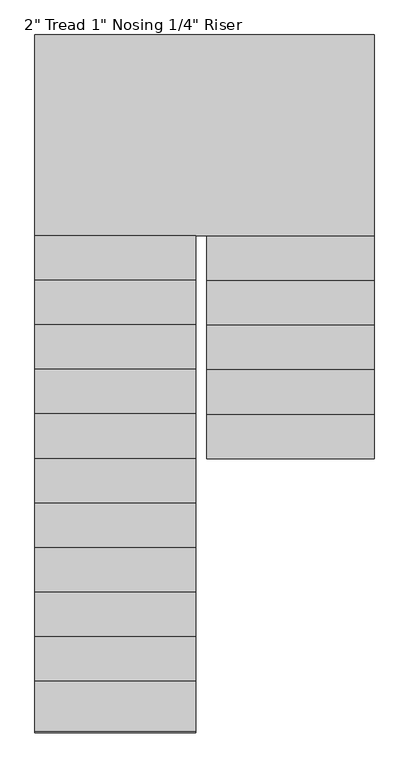
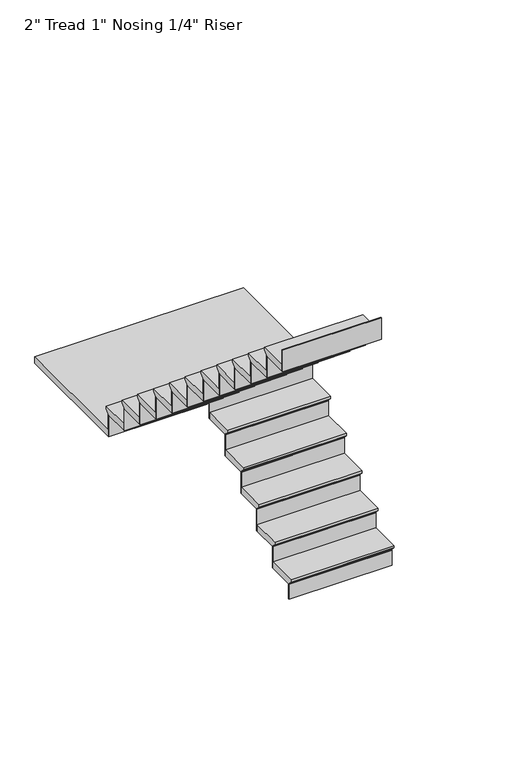
"""IFC4 building model written with IfcOpenShell, lengths in millimetres: stair flight geometry."""

from ifc_helpers import new_model, si_unit, origin, place, context, project, spatial, faceted_brep, source, transform, mapped, element, save


def stair_flight_ae003db1(model_context):
    return source(origin(), model_context, "Body", "Brep", [
        faceted_brep([(-3749.597125, 2714.6319226, 18285.8833333), (-3749.597125, 2714.6319226, 18304.9333333), (-4512.2136682, 2714.6319226, 18304.9333333), (-4512.2136682, 2714.6319226, 18285.8833333), (-3749.597125, 2740.0319226, 18260.4833333), (-4512.2136682, 2740.0319226, 18260.4833333), (-3749.597125, 2943.2319226, 18304.9333333), (-4512.2136682, 2943.2319226, 18304.9333333), (-4512.2136682, 2740.0319226, 18254.1333333), (-4512.2136682, 2943.2319226, 18254.1333333), (-3749.597125, 2943.2319226, 18254.1333333), (-3749.597125, 2740.0319226, 18254.1333333)], [[[0, 1, 2, 3]], [[4, 0, 3, 5]], [[2, 1, 6, 7]], [[8, 9, 10, 11]], [[2, 7, 9, 8, 5, 3]], [[8, 11, 4, 5]], [[6, 1, 0, 4, 11, 10]], [[7, 6, 10, 9]]]),
        faceted_brep([(-3749.597125, 2740.0319226, 18254.1333333), (-3749.597125, 2740.0319226, 18135.6), (-3749.597125, 2746.3819226, 18135.6), (-3749.597125, 2746.3819226, 18254.1333333), (-4512.2136682, 2740.0319226, 18254.1333333), (-4512.2136682, 2746.3819226, 18254.1333333), (-4512.2136682, 2746.3819226, 18135.6), (-4512.2136682, 2740.0319226, 18135.6)], [[[0, 1, 2, 3]], [[4, 5, 6, 7]], [[1, 0, 4, 7]], [[2, 1, 7, 6]], [[3, 2, 6, 5]], [[0, 3, 5, 4]]]),
        faceted_brep([(-3749.597125, 2943.2319226, 18423.4666667), (-3749.597125, 2943.2319226, 18254.1333333), (-3749.597125, 2949.5819226, 18254.1333333), (-3749.597125, 2949.5819226, 18423.4666667), (-4512.2136682, 2943.2319226, 18423.4666667), (-4512.2136682, 2949.5819226, 18423.4666667), (-4512.2136682, 2949.5819226, 18254.1333333), (-4512.2136682, 2943.2319226, 18254.1333333)], [[[0, 1, 2, 3]], [[4, 5, 6, 7]], [[1, 0, 4, 7]], [[2, 1, 7, 6]], [[3, 2, 6, 5]], [[0, 3, 5, 4]]]),
        faceted_brep([(-4512.2136682, 2917.8319226, 18474.2666667), (-3749.597125, 2917.8319226, 18474.2666667), (-3749.597125, 3146.4319226, 18474.2666667), (-4512.2136682, 3146.4319226, 18474.2666667), (-4512.2136682, 2943.2319226, 18423.4666667), (-4512.2136682, 3146.4319226, 18423.4666667), (-3749.597125, 3146.4319226, 18423.4666667), (-3749.597125, 2943.2319226, 18423.4666667), (-4512.2136682, 2943.2319226, 18429.8166667), (-4512.2136682, 2917.8319226, 18455.2166667), (-3749.597125, 2943.2319226, 18429.8166667), (-3749.597125, 2917.8319226, 18455.2166667)], [[[0, 1, 2, 3]], [[4, 5, 6, 7]], [[0, 3, 5, 4, 8, 9]], [[4, 7, 10, 8]], [[2, 1, 11, 10, 7, 6]], [[3, 2, 6, 5]], [[11, 1, 0, 9]], [[10, 11, 9, 8]]]),
        faceted_brep([(-3749.597125, 3146.4319226, 18592.8), (-3749.597125, 3146.4319226, 18423.4666667), (-3749.597125, 3152.7819226, 18423.4666667), (-3749.597125, 3152.7819226, 18592.8), (-4512.2136682, 3146.4319226, 18592.8), (-4512.2136682, 3152.7819226, 18592.8), (-4512.2136682, 3152.7819226, 18423.4666667), (-4512.2136682, 3146.4319226, 18423.4666667)], [[[0, 1, 2, 3]], [[4, 5, 6, 7]], [[1, 0, 4, 7]], [[2, 1, 7, 6]], [[3, 2, 6, 5]], [[0, 3, 5, 4]]]),
        faceted_brep([(-4512.2136682, 3121.0319226, 18643.6), (-3749.597125, 3121.0319226, 18643.6), (-3749.597125, 3349.6319226, 18643.6), (-4512.2136682, 3349.6319226, 18643.6), (-4512.2136682, 3146.4319226, 18592.8), (-4512.2136682, 3349.6319226, 18592.8), (-3749.597125, 3349.6319226, 18592.8), (-3749.597125, 3146.4319226, 18592.8), (-4512.2136682, 3146.4319226, 18599.15), (-4512.2136682, 3121.0319226, 18624.55), (-3749.597125, 3146.4319226, 18599.15), (-3749.597125, 3121.0319226, 18624.55)], [[[0, 1, 2, 3]], [[4, 5, 6, 7]], [[0, 3, 5, 4, 8, 9]], [[4, 7, 10, 8]], [[2, 1, 11, 10, 7, 6]], [[3, 2, 6, 5]], [[11, 1, 0, 9]], [[10, 11, 9, 8]]]),
        faceted_brep([(-3749.597125, 3349.6319226, 18762.1333333), (-3749.597125, 3349.6319226, 18592.8), (-3749.597125, 3355.9819226, 18592.8), (-3749.597125, 3355.9819226, 18762.1333333), (-4512.2136682, 3349.6319226, 18762.1333333), (-4512.2136682, 3355.9819226, 18762.1333333), (-4512.2136682, 3355.9819226, 18592.8), (-4512.2136682, 3349.6319226, 18592.8)], [[[0, 1, 2, 3]], [[4, 5, 6, 7]], [[1, 0, 4, 7]], [[2, 1, 7, 6]], [[3, 2, 6, 5]], [[0, 3, 5, 4]]]),
        faceted_brep([(-4512.2136682, 3324.2319226, 18812.9333333), (-3749.597125, 3324.2319226, 18812.9333333), (-3749.597125, 3552.8319226, 18812.9333333), (-4512.2136682, 3552.8319226, 18812.9333333), (-4512.2136682, 3349.6319226, 18762.1333333), (-4512.2136682, 3552.8319226, 18762.1333333), (-3749.597125, 3552.8319226, 18762.1333333), (-3749.597125, 3349.6319226, 18762.1333333), (-4512.2136682, 3349.6319226, 18768.4833333), (-4512.2136682, 3324.2319226, 18793.8833333), (-3749.597125, 3349.6319226, 18768.4833333), (-3749.597125, 3324.2319226, 18793.8833333)], [[[0, 1, 2, 3]], [[4, 5, 6, 7]], [[0, 3, 5, 4, 8, 9]], [[4, 7, 10, 8]], [[2, 1, 11, 10, 7, 6]], [[3, 2, 6, 5]], [[11, 1, 0, 9]], [[10, 11, 9, 8]]]),
        faceted_brep([(-3749.597125, 3552.8319226, 18931.4666667), (-3749.597125, 3552.8319226, 18762.1333333), (-3749.597125, 3559.1819226, 18762.1333333), (-3749.597125, 3559.1819226, 18931.4666667), (-4512.2136682, 3552.8319226, 18931.4666667), (-4512.2136682, 3559.1819226, 18931.4666667), (-4512.2136682, 3559.1819226, 18762.1333333), (-4512.2136682, 3552.8319226, 18762.1333333)], [[[0, 1, 2, 3]], [[4, 5, 6, 7]], [[1, 0, 4, 7]], [[2, 1, 7, 6]], [[3, 2, 6, 5]], [[0, 3, 5, 4]]]),
        faceted_brep([(-4512.2136682, 3527.4319226, 18982.2666667), (-3749.597125, 3527.4319226, 18982.2666667), (-3749.597125, 3756.0319226, 18982.2666667), (-4512.2136682, 3756.0319226, 18982.2666667), (-4512.2136682, 3552.8319226, 18931.4666667), (-4512.2136682, 3756.0319226, 18931.4666667), (-3749.597125, 3756.0319226, 18931.4666667), (-3749.597125, 3552.8319226, 18931.4666667), (-4512.2136682, 3552.8319226, 18937.8166667), (-4512.2136682, 3527.4319226, 18963.2166667), (-3749.597125, 3552.8319226, 18937.8166667), (-3749.597125, 3527.4319226, 18963.2166667)], [[[0, 1, 2, 3]], [[4, 5, 6, 7]], [[0, 3, 5, 4, 8, 9]], [[4, 7, 10, 8]], [[2, 1, 11, 10, 7, 6]], [[3, 2, 6, 5]], [[11, 1, 0, 9]], [[10, 11, 9, 8]]]),
        faceted_brep([(-3749.597125, 3756.0319226, 19100.8), (-3749.597125, 3756.0319226, 18931.4666667), (-3749.597125, 3762.3819226, 18931.4666667), (-3749.597125, 3762.3819226, 19100.8), (-4512.2136682, 3756.0319226, 19100.8), (-4512.2136682, 3762.3819226, 19100.8), (-4512.2136682, 3762.3819226, 18931.4666667), (-4512.2136682, 3756.0319226, 18931.4666667)], [[[0, 1, 2, 3]], [[4, 5, 6, 7]], [[1, 0, 4, 7]], [[2, 1, 7, 6]], [[3, 2, 6, 5]], [[0, 3, 5, 4]]]),
        faceted_brep([(-4563.0136682, 3705.2319226, 19151.6), (-4563.0136682, 3730.6319226, 19151.6), (-3749.597125, 3730.6319226, 19151.6), (-3749.597125, 4645.0319226, 19151.6), (-5295.0246464, 4645.0319226, 19151.6), (-5295.0246464, 3705.2319226, 19151.6), (-4563.0136682, 3730.6319226, 19100.8), (-4563.0136682, 3705.2319226, 19100.8), (-5295.0246464, 3705.2319226, 19100.8), (-5295.0246464, 4645.0319226, 19100.8), (-3749.597125, 4645.0319226, 19100.8), (-3749.597125, 3756.0319226, 19100.8), (-4512.2136682, 3756.0319226, 19100.8), (-4512.2136682, 3730.6319226, 19100.8), (-4512.2136682, 3730.6319226, 19132.55), (-3749.597125, 3730.6319226, 19132.55), (-4512.2136682, 3756.0319226, 19107.15), (-3749.597125, 3756.0319226, 19107.15)], [[[0, 1, 2, 3, 4, 5]], [[6, 7, 8, 9, 10, 11, 12, 13]], [[1, 0, 7, 6]], [[2, 1, 6, 13, 14, 15]], [[13, 12, 16, 14]], [[12, 11, 17, 16]], [[3, 2, 15, 17, 11, 10]], [[4, 3, 10, 9]], [[5, 4, 9, 8]], [[0, 5, 8, 7]], [[17, 15, 14, 16]]]),
        faceted_brep([(-5295.0246464, 3705.2319226, 19270.1333333), (-5295.0246464, 3705.2319226, 19100.8), (-5295.0246464, 3698.8819226, 19100.8), (-5295.0246464, 3698.8819226, 19270.1333333), (-4563.0136682, 3705.2319226, 19270.1333333), (-4563.0136682, 3698.8819226, 19270.1333333), (-4563.0136682, 3698.8819226, 19100.8), (-4563.0136682, 3705.2319226, 19100.8)], [[[0, 1, 2, 3]], [[4, 5, 6, 7]], [[1, 0, 4, 7]], [[2, 1, 7, 6]], [[3, 2, 6, 5]], [[0, 3, 5, 4]]]),
        faceted_brep([(-4563.0136682, 3730.6319226, 19320.9333333), (-5295.0246464, 3730.6319226, 19320.9333333), (-5295.0246464, 3502.0319226, 19320.9333333), (-4563.0136682, 3502.0319226, 19320.9333333), (-4563.0136682, 3705.2319226, 19270.1333333), (-4563.0136682, 3502.0319226, 19270.1333333), (-5295.0246464, 3502.0319226, 19270.1333333), (-5295.0246464, 3705.2319226, 19270.1333333), (-4563.0136682, 3705.2319226, 19276.4833333), (-4563.0136682, 3730.6319226, 19301.8833333), (-5295.0246464, 3705.2319226, 19276.4833333), (-5295.0246464, 3730.6319226, 19301.8833333)], [[[0, 1, 2, 3]], [[4, 5, 6, 7]], [[0, 3, 5, 4, 8, 9]], [[4, 7, 10, 8]], [[2, 1, 11, 10, 7, 6]], [[3, 2, 6, 5]], [[11, 1, 0, 9]], [[10, 11, 9, 8]]]),
        faceted_brep([(-5295.0246464, 3502.0319226, 19439.4666667), (-5295.0246464, 3502.0319226, 19270.1333333), (-5295.0246464, 3495.6819226, 19270.1333333), (-5295.0246464, 3495.6819226, 19439.4666667), (-4563.0136682, 3502.0319226, 19439.4666667), (-4563.0136682, 3495.6819226, 19439.4666667), (-4563.0136682, 3495.6819226, 19270.1333333), (-4563.0136682, 3502.0319226, 19270.1333333)], [[[0, 1, 2, 3]], [[4, 5, 6, 7]], [[1, 0, 4, 7]], [[2, 1, 7, 6]], [[3, 2, 6, 5]], [[0, 3, 5, 4]]]),
        faceted_brep([(-4563.0136682, 3527.4319226, 19490.2666667), (-5295.0246464, 3527.4319226, 19490.2666667), (-5295.0246464, 3298.8319226, 19490.2666667), (-4563.0136682, 3298.8319226, 19490.2666667), (-4563.0136682, 3502.0319226, 19439.4666667), (-4563.0136682, 3298.8319226, 19439.4666667), (-5295.0246464, 3298.8319226, 19439.4666667), (-5295.0246464, 3502.0319226, 19439.4666667), (-4563.0136682, 3502.0319226, 19445.8166667), (-4563.0136682, 3527.4319226, 19471.2166667), (-5295.0246464, 3502.0319226, 19445.8166667), (-5295.0246464, 3527.4319226, 19471.2166667)], [[[0, 1, 2, 3]], [[4, 5, 6, 7]], [[0, 3, 5, 4, 8, 9]], [[4, 7, 10, 8]], [[2, 1, 11, 10, 7, 6]], [[3, 2, 6, 5]], [[11, 1, 0, 9]], [[10, 11, 9, 8]]]),
        faceted_brep([(-5295.0246464, 3298.8319226, 19608.8), (-5295.0246464, 3298.8319226, 19439.4666667), (-5295.0246464, 3292.4819226, 19439.4666667), (-5295.0246464, 3292.4819226, 19608.8), (-4563.0136682, 3298.8319226, 19608.8), (-4563.0136682, 3292.4819226, 19608.8), (-4563.0136682, 3292.4819226, 19439.4666667), (-4563.0136682, 3298.8319226, 19439.4666667)], [[[0, 1, 2, 3]], [[4, 5, 6, 7]], [[1, 0, 4, 7]], [[2, 1, 7, 6]], [[3, 2, 6, 5]], [[0, 3, 5, 4]]]),
        faceted_brep([(-4563.0136682, 3324.2319226, 19659.6), (-5295.0246464, 3324.2319226, 19659.6), (-5295.0246464, 3095.6319226, 19659.6), (-4563.0136682, 3095.6319226, 19659.6), (-4563.0136682, 3298.8319226, 19608.8), (-4563.0136682, 3095.6319226, 19608.8), (-5295.0246464, 3095.6319226, 19608.8), (-5295.0246464, 3298.8319226, 19608.8), (-4563.0136682, 3298.8319226, 19615.15), (-4563.0136682, 3324.2319226, 19640.55), (-5295.0246464, 3298.8319226, 19615.15), (-5295.0246464, 3324.2319226, 19640.55)], [[[0, 1, 2, 3]], [[4, 5, 6, 7]], [[0, 3, 5, 4, 8, 9]], [[4, 7, 10, 8]], [[2, 1, 11, 10, 7, 6]], [[3, 2, 6, 5]], [[11, 1, 0, 9]], [[10, 11, 9, 8]]]),
        faceted_brep([(-5295.0246464, 3095.6319226, 19778.1333333), (-5295.0246464, 3095.6319226, 19608.8), (-5295.0246464, 3089.2819226, 19608.8), (-5295.0246464, 3089.2819226, 19778.1333333), (-4563.0136682, 3095.6319226, 19778.1333333), (-4563.0136682, 3089.2819226, 19778.1333333), (-4563.0136682, 3089.2819226, 19608.8), (-4563.0136682, 3095.6319226, 19608.8)], [[[0, 1, 2, 3]], [[4, 5, 6, 7]], [[1, 0, 4, 7]], [[2, 1, 7, 6]], [[3, 2, 6, 5]], [[0, 3, 5, 4]]]),
        faceted_brep([(-4563.0136682, 3121.0319226, 19828.9333333), (-5295.0246464, 3121.0319226, 19828.9333333), (-5295.0246464, 2892.4319226, 19828.9333333), (-4563.0136682, 2892.4319226, 19828.9333333), (-4563.0136682, 3095.6319226, 19778.1333333), (-4563.0136682, 2892.4319226, 19778.1333333), (-5295.0246464, 2892.4319226, 19778.1333333), (-5295.0246464, 3095.6319226, 19778.1333333), (-4563.0136682, 3095.6319226, 19784.4833333), (-4563.0136682, 3121.0319226, 19809.8833333), (-5295.0246464, 3095.6319226, 19784.4833333), (-5295.0246464, 3121.0319226, 19809.8833333)], [[[0, 1, 2, 3]], [[4, 5, 6, 7]], [[0, 3, 5, 4, 8, 9]], [[4, 7, 10, 8]], [[2, 1, 11, 10, 7, 6]], [[3, 2, 6, 5]], [[11, 1, 0, 9]], [[10, 11, 9, 8]]]),
        faceted_brep([(-5295.0246464, 2892.4319226, 19947.4666667), (-5295.0246464, 2892.4319226, 19778.1333333), (-5295.0246464, 2886.0819226, 19778.1333333), (-5295.0246464, 2886.0819226, 19947.4666667), (-4563.0136682, 2892.4319226, 19947.4666667), (-4563.0136682, 2886.0819226, 19947.4666667), (-4563.0136682, 2886.0819226, 19778.1333333), (-4563.0136682, 2892.4319226, 19778.1333333)], [[[0, 1, 2, 3]], [[4, 5, 6, 7]], [[1, 0, 4, 7]], [[2, 1, 7, 6]], [[3, 2, 6, 5]], [[0, 3, 5, 4]]]),
        faceted_brep([(-4563.0136682, 2917.8319226, 19998.2666667), (-5295.0246464, 2917.8319226, 19998.2666667), (-5295.0246464, 2689.2319226, 19998.2666667), (-4563.0136682, 2689.2319226, 19998.2666667), (-4563.0136682, 2892.4319226, 19947.4666667), (-4563.0136682, 2689.2319226, 19947.4666667), (-5295.0246464, 2689.2319226, 19947.4666667), (-5295.0246464, 2892.4319226, 19947.4666667), (-4563.0136682, 2892.4319226, 19953.8166667), (-4563.0136682, 2917.8319226, 19979.2166667), (-5295.0246464, 2892.4319226, 19953.8166667), (-5295.0246464, 2917.8319226, 19979.2166667)], [[[0, 1, 2, 3]], [[4, 5, 6, 7]], [[0, 3, 5, 4, 8, 9]], [[4, 7, 10, 8]], [[2, 1, 11, 10, 7, 6]], [[3, 2, 6, 5]], [[11, 1, 0, 9]], [[10, 11, 9, 8]]]),
        faceted_brep([(-5295.0246464, 2689.2319226, 20116.8), (-5295.0246464, 2689.2319226, 19947.4666667), (-5295.0246464, 2682.8819226, 19947.4666667), (-5295.0246464, 2682.8819226, 20116.8), (-4563.0136682, 2689.2319226, 20116.8), (-4563.0136682, 2682.8819226, 20116.8), (-4563.0136682, 2682.8819226, 19947.4666667), (-4563.0136682, 2689.2319226, 19947.4666667)], [[[0, 1, 2, 3]], [[4, 5, 6, 7]], [[1, 0, 4, 7]], [[2, 1, 7, 6]], [[3, 2, 6, 5]], [[0, 3, 5, 4]]]),
        faceted_brep([(-4563.0136682, 2714.6319226, 20167.6), (-5295.0246464, 2714.6319226, 20167.6), (-5295.0246464, 2486.0319226, 20167.6), (-4563.0136682, 2486.0319226, 20167.6), (-4563.0136682, 2689.2319226, 20116.8), (-4563.0136682, 2486.0319226, 20116.8), (-5295.0246464, 2486.0319226, 20116.8), (-5295.0246464, 2689.2319226, 20116.8), (-4563.0136682, 2689.2319226, 20123.15), (-4563.0136682, 2714.6319226, 20148.55), (-5295.0246464, 2689.2319226, 20123.15), (-5295.0246464, 2714.6319226, 20148.55)], [[[0, 1, 2, 3]], [[4, 5, 6, 7]], [[0, 3, 5, 4, 8, 9]], [[4, 7, 10, 8]], [[2, 1, 11, 10, 7, 6]], [[3, 2, 6, 5]], [[11, 1, 0, 9]], [[10, 11, 9, 8]]]),
        faceted_brep([(-5295.0246464, 2486.0319226, 20286.1333333), (-5295.0246464, 2486.0319226, 20116.8), (-5295.0246464, 2479.6819226, 20116.8), (-5295.0246464, 2479.6819226, 20286.1333333), (-4563.0136682, 2486.0319226, 20286.1333333), (-4563.0136682, 2479.6819226, 20286.1333333), (-4563.0136682, 2479.6819226, 20116.8), (-4563.0136682, 2486.0319226, 20116.8)], [[[0, 1, 2, 3]], [[4, 5, 6, 7]], [[1, 0, 4, 7]], [[2, 1, 7, 6]], [[3, 2, 6, 5]], [[0, 3, 5, 4]]]),
        faceted_brep([(-4563.0136682, 2511.4319226, 20336.9333333), (-5295.0246464, 2511.4319226, 20336.9333333), (-5295.0246464, 2282.8319226, 20336.9333333), (-4563.0136682, 2282.8319226, 20336.9333333), (-4563.0136682, 2486.0319226, 20286.1333333), (-4563.0136682, 2282.8319226, 20286.1333333), (-5295.0246464, 2282.8319226, 20286.1333333), (-5295.0246464, 2486.0319226, 20286.1333333), (-4563.0136682, 2486.0319226, 20292.4833333), (-4563.0136682, 2511.4319226, 20317.8833333), (-5295.0246464, 2486.0319226, 20292.4833333), (-5295.0246464, 2511.4319226, 20317.8833333)], [[[0, 1, 2, 3]], [[4, 5, 6, 7]], [[0, 3, 5, 4, 8, 9]], [[4, 7, 10, 8]], [[2, 1, 11, 10, 7, 6]], [[3, 2, 6, 5]], [[11, 1, 0, 9]], [[10, 11, 9, 8]]]),
        faceted_brep([(-5295.0246464, 2282.8319226, 20455.4666667), (-5295.0246464, 2282.8319226, 20286.1333333), (-5295.0246464, 2276.4819226, 20286.1333333), (-5295.0246464, 2276.4819226, 20455.4666667), (-4563.0136682, 2282.8319226, 20455.4666667), (-4563.0136682, 2276.4819226, 20455.4666667), (-4563.0136682, 2276.4819226, 20286.1333333), (-4563.0136682, 2282.8319226, 20286.1333333)], [[[0, 1, 2, 3]], [[4, 5, 6, 7]], [[1, 0, 4, 7]], [[2, 1, 7, 6]], [[3, 2, 6, 5]], [[0, 3, 5, 4]]]),
        faceted_brep([(-4563.0136682, 2308.2319226, 20506.2666667), (-5295.0246464, 2308.2319226, 20506.2666667), (-5295.0246464, 2079.6319226, 20506.2666667), (-4563.0136682, 2079.6319226, 20506.2666667), (-4563.0136682, 2282.8319226, 20455.4666667), (-4563.0136682, 2079.6319226, 20455.4666667), (-5295.0246464, 2079.6319226, 20455.4666667), (-5295.0246464, 2282.8319226, 20455.4666667), (-4563.0136682, 2282.8319226, 20461.8166667), (-4563.0136682, 2308.2319226, 20487.2166667), (-5295.0246464, 2282.8319226, 20461.8166667), (-5295.0246464, 2308.2319226, 20487.2166667)], [[[0, 1, 2, 3]], [[4, 5, 6, 7]], [[0, 3, 5, 4, 8, 9]], [[4, 7, 10, 8]], [[2, 1, 11, 10, 7, 6]], [[3, 2, 6, 5]], [[11, 1, 0, 9]], [[10, 11, 9, 8]]]),
        faceted_brep([(-5295.0246464, 2079.6319226, 20624.8), (-5295.0246464, 2079.6319226, 20455.4666667), (-5295.0246464, 2073.2819226, 20455.4666667), (-5295.0246464, 2073.2819226, 20624.8), (-4563.0136682, 2079.6319226, 20624.8), (-4563.0136682, 2073.2819226, 20624.8), (-4563.0136682, 2073.2819226, 20455.4666667), (-4563.0136682, 2079.6319226, 20455.4666667)], [[[0, 1, 2, 3]], [[4, 5, 6, 7]], [[1, 0, 4, 7]], [[2, 1, 7, 6]], [[3, 2, 6, 5]], [[0, 3, 5, 4]]]),
        faceted_brep([(-4563.0136682, 2105.0319226, 20675.6), (-5295.0246464, 2105.0319226, 20675.6), (-5295.0246464, 1876.4319226, 20675.6), (-4563.0136682, 1876.4319226, 20675.6), (-4563.0136682, 2079.6319226, 20624.8), (-4563.0136682, 1876.4319226, 20624.8), (-5295.0246464, 1876.4319226, 20624.8), (-5295.0246464, 2079.6319226, 20624.8), (-4563.0136682, 2079.6319226, 20631.15), (-4563.0136682, 2105.0319226, 20656.55), (-5295.0246464, 2079.6319226, 20631.15), (-5295.0246464, 2105.0319226, 20656.55)], [[[0, 1, 2, 3]], [[4, 5, 6, 7]], [[0, 3, 5, 4, 8, 9]], [[4, 7, 10, 8]], [[2, 1, 11, 10, 7, 6]], [[3, 2, 6, 5]], [[11, 1, 0, 9]], [[10, 11, 9, 8]]]),
        faceted_brep([(-5295.0246464, 1876.4319226, 20794.1333333), (-5295.0246464, 1876.4319226, 20624.8), (-5295.0246464, 1870.0819226, 20624.8), (-5295.0246464, 1870.0819226, 20794.1333333), (-4563.0136682, 1876.4319226, 20794.1333333), (-4563.0136682, 1870.0819226, 20794.1333333), (-4563.0136682, 1870.0819226, 20624.8), (-4563.0136682, 1876.4319226, 20624.8)], [[[0, 1, 2, 3]], [[4, 5, 6, 7]], [[1, 0, 4, 7]], [[2, 1, 7, 6]], [[3, 2, 6, 5]], [[0, 3, 5, 4]]]),
        faceted_brep([(-4563.0136682, 1901.8319226, 20844.9333333), (-5295.0246464, 1901.8319226, 20844.9333333), (-5295.0246464, 1673.2319226, 20844.9333333), (-4563.0136682, 1673.2319226, 20844.9333333), (-4563.0136682, 1876.4319226, 20794.1333333), (-4563.0136682, 1673.2319226, 20794.1333333), (-5295.0246464, 1673.2319226, 20794.1333333), (-5295.0246464, 1876.4319226, 20794.1333333), (-4563.0136682, 1876.4319226, 20800.4833333), (-4563.0136682, 1901.8319226, 20825.8833333), (-5295.0246464, 1876.4319226, 20800.4833333), (-5295.0246464, 1901.8319226, 20825.8833333)], [[[0, 1, 2, 3]], [[4, 5, 6, 7]], [[0, 3, 5, 4, 8, 9]], [[4, 7, 10, 8]], [[2, 1, 11, 10, 7, 6]], [[3, 2, 6, 5]], [[11, 1, 0, 9]], [[10, 11, 9, 8]]]),
        faceted_brep([(-5295.0246464, 1673.2319226, 20963.4666667), (-5295.0246464, 1673.2319226, 20794.1333333), (-5295.0246464, 1666.8819226, 20794.1333333), (-5295.0246464, 1666.8819226, 20963.4666667), (-4563.0136682, 1673.2319226, 20963.4666667), (-4563.0136682, 1666.8819226, 20963.4666667), (-4563.0136682, 1666.8819226, 20794.1333333), (-4563.0136682, 1673.2319226, 20794.1333333)], [[[0, 1, 2, 3]], [[4, 5, 6, 7]], [[1, 0, 4, 7]], [[2, 1, 7, 6]], [[3, 2, 6, 5]], [[0, 3, 5, 4]]]),
        faceted_brep([(-4563.0136682, 1698.6319226, 21014.2666667), (-5295.0246464, 1698.6319226, 21014.2666667), (-5295.0246464, 1470.0319226, 21014.2666667), (-4563.0136682, 1470.0319226, 21014.2666667), (-4563.0136682, 1673.2319226, 20963.4666667), (-4563.0136682, 1470.0319226, 20963.4666667), (-5295.0246464, 1470.0319226, 20963.4666667), (-5295.0246464, 1673.2319226, 20963.4666667), (-4563.0136682, 1673.2319226, 20969.8166667), (-4563.0136682, 1698.6319226, 20995.2166667), (-5295.0246464, 1673.2319226, 20969.8166667), (-5295.0246464, 1698.6319226, 20995.2166667)], [[[0, 1, 2, 3]], [[4, 5, 6, 7]], [[0, 3, 5, 4, 8, 9]], [[4, 7, 10, 8]], [[2, 1, 11, 10, 7, 6]], [[3, 2, 6, 5]], [[11, 1, 0, 9]], [[10, 11, 9, 8]]]),
        faceted_brep([(-5295.0246464, 1470.0319226, 21132.8), (-5295.0246464, 1470.0319226, 20963.4666667), (-5295.0246464, 1463.6819226, 20963.4666667), (-5295.0246464, 1463.6819226, 21132.8), (-4563.0136682, 1470.0319226, 21132.8), (-4563.0136682, 1463.6819226, 21132.8), (-4563.0136682, 1463.6819226, 20963.4666667), (-4563.0136682, 1470.0319226, 20963.4666667)], [[[0, 1, 2, 3]], [[4, 5, 6, 7]], [[1, 0, 4, 7]], [[2, 1, 7, 6]], [[3, 2, 6, 5]], [[0, 3, 5, 4]]]),
    ])


if __name__ == "__main__":
    model = new_model("IFC4")
    model_context = context("Model", 3, world=origin())
    ifc_project = project(units=[si_unit("LENGTHUNIT", "METRE", prefix="MILLI")], contexts=[model_context])
    site = spatial("IfcSite", under=ifc_project)
    building = spatial("IfcBuilding", under=site)
    placement = place(None, origin())
    stair_flight_shape = stair_flight_ae003db1(model_context)
    element("IfcStairFlight", 1, ObjectType="2\" Tread 1\" Nosing 1/4\" Riser", at=placement, inside=building, context=model_context, shape_type="MappedRepresentation", body=[
        mapped(stair_flight_shape, transform((0.0, 0.0, 0.0), x_axis=(1.0, 0.0, 0.0), y_axis=(0.0, 1.0, 0.0), z_axis=(0.0, 0.0, 1.0))),
    ])
    save(model, "model.ifc")
